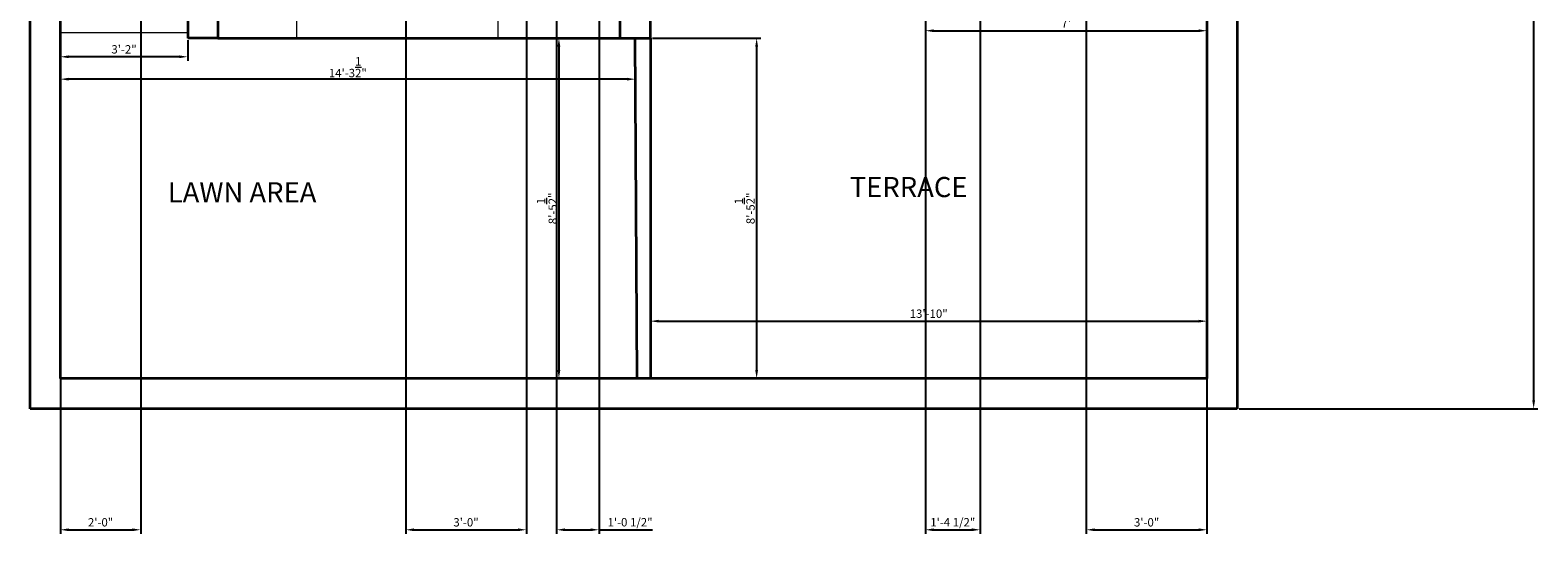
# Model space of a CAD drawing. Units: inches. Extents: x 2178 to 2667, y 1439 to 2239.
# Tile 1 of 5: x 2218 to 2667, y 1439 to 1590. Entities that reach past the tile are written whole.
import ezdxf

# ---------------------------------------------------------------- set-up
doc = ezdxf.new("R2010")
doc.units = ezdxf.units.IN
for name, color, linetype, lineweight in [('A-ANNO-DIMS', 2, 'Continuous', 18), ('A-AREA-IDEN', 7, 'Continuous', 18), ('A-FLOR-PATT', 252, 'Continuous', 13), ('A-GLAZ', 4, 'Continuous', 18), ('A-WALL', 7, 'Continuous', 35)]:
    doc.layers.add(name, color=color, linetype=linetype, lineweight=lineweight)
doc.styles.get("Standard").update_dxf_attribs({"font": 'arial.ttf'})
doc.dimstyles.new('Copy of ISO-25', dxfattribs={"dimtxt": 2.5, "dimasz": 2.5, "dimexe": 1.25, "dimexo": 0.625, "dimtad": 1, "dimdec": 1, "dimlunit": 4, "dimtxsty": 'Standard', "dimcen": 2.5, "dimadec": 0, "dimazin": 0, "dimtfac": 1, "dimtdec": 1, "dimtmove": 0, "dimatfit": 3, "dimfxl": 1, "dimarcsym": 0})

# ---------------------------------------------------------------- blocks, each defined once
blk = doc.blocks.new('*D25')
at = {"layer": 'A-ANNO-DIMS', "color": 0, "lineweight": -2, "transparency": 16777216}
for p, q in [((2226.53, 1586.91), (2226.53, 1574.05)), ((2398.03, 1586.91), (2398.03, 1574.05)), ((2395.53, 1575.3), (2229.03, 1575.3))]:
    blk.add_line(p, q, dxfattribs=at)
at = {"layer": 'A-ANNO-DIMS', "color": 0, "transparency": 16777216}
for points in [[(2229.03, 1575.72), (2229.03, 1574.89), (2226.53, 1575.3)], [(2395.53, 1575.72), (2395.53, 1574.89), (2398.03, 1575.3)]]:
    blk.add_solid(points, dxfattribs=at)
at = {"layer": 'Defpoints', "color": 0, "transparency": 16777216}
for p in [(2226.53, 1587.53), (2398.03, 1587.53), (2226.53, 1575.3)]:
    blk.add_point(p, dxfattribs=at)
at = {"layer": 'A-ANNO-DIMS', "color": 0, "transparency": 16777216, "insert": (2312.28, 1578.88), "char_height": 2.5, "attachment_point": 5}
blk.add_mtext('14\'-3{\\H1x;\\S1/2;}"', dxfattribs=at)
blk = doc.blocks.new('*D26')
at = {"layer": 'A-ANNO-DIMS', "color": 0, "lineweight": -2, "transparency": 16777216}
for p, q in [((2397.4, 1587.53), (2373.98, 1587.53)), ((2375.23, 1585.03), (2375.23, 1488.53)), ((2397.9, 1486.03), (2373.98, 1486.03))]:
    blk.add_line(p, q, dxfattribs=at)
at = {"layer": 'A-ANNO-DIMS', "color": 0, "transparency": 16777216}
for points in [[(2374.82, 1585.03), (2375.65, 1585.03), (2375.23, 1587.53)], [(2374.82, 1488.53), (2375.65, 1488.53), (2375.23, 1486.03)]]:
    blk.add_solid(points, dxfattribs=at)
at = {"layer": 'Defpoints', "color": 0, "transparency": 16777216}
for p in [(2398.03, 1587.53), (2375.23, 1486.03), (2398.53, 1486.03)]:
    blk.add_point(p, dxfattribs=at)
at = {"layer": 'A-ANNO-DIMS', "color": 0, "transparency": 16777216, "insert": (2371.66, 1536.78), "char_height": 2.5, "attachment_point": 5, "rotation": 90}
blk.add_mtext('8\'-5{\\H1x;\\S1/2;}"', dxfattribs=at)
blk = doc.blocks.new('*D27')
at = {"layer": 'A-ANNO-DIMS', "color": 0, "lineweight": -2, "transparency": 16777216}
for p, q in [((2402.53, 1486.66), (2402.53, 1504.39)), ((2405.03, 1503.14), (2566.03, 1503.14)), ((2568.53, 1486.66), (2568.53, 1504.39))]:
    blk.add_line(p, q, dxfattribs=at)
at = {"layer": 'A-ANNO-DIMS', "color": 0, "transparency": 16777216}
for points in [[(2405.03, 1503.56), (2405.03, 1502.73), (2402.53, 1503.14)], [(2566.03, 1503.56), (2566.03, 1502.73), (2568.53, 1503.14)]]:
    blk.add_solid(points, dxfattribs=at)
at = {"layer": 'Defpoints', "color": 0, "transparency": 16777216}
for p in [(2568.53, 1503.14), (2402.53, 1486.03), (2568.53, 1486.03)]:
    blk.add_point(p, dxfattribs=at)
at = {"layer": 'A-ANNO-DIMS', "color": 0, "transparency": 16777216, "insert": (2485.53, 1505.05), "char_height": 2.5, "attachment_point": 5}
blk.add_mtext('13\'-10"', dxfattribs=at)
blk = doc.blocks.new('*D28')
at = {"layer": 'A-ANNO-DIMS', "color": 0, "lineweight": -2, "transparency": 16777216}
for p, q in [((2403.15, 1587.53), (2435.47, 1587.53)), ((2434.22, 1585.03), (2434.22, 1488.53)), ((2403.15, 1486.03), (2435.47, 1486.03))]:
    blk.add_line(p, q, dxfattribs=at)
at = {"layer": 'A-ANNO-DIMS', "color": 0, "transparency": 16777216}
for points in [[(2433.8, 1585.03), (2434.63, 1585.03), (2434.22, 1587.53)], [(2433.8, 1488.53), (2434.63, 1488.53), (2434.22, 1486.03)]]:
    blk.add_solid(points, dxfattribs=at)
at = {"layer": 'Defpoints', "color": 0, "transparency": 16777216}
for p in [(2402.53, 1587.53), (2402.53, 1486.03), (2434.22, 1486.03)]:
    blk.add_point(p, dxfattribs=at)
at = {"layer": 'A-ANNO-DIMS', "color": 0, "transparency": 16777216, "insert": (2430.64, 1536.78), "char_height": 2.5, "attachment_point": 5, "rotation": 90}
blk.add_mtext('8\'-5{\\H1x;\\S1/2;}"', dxfattribs=at)
blk = doc.blocks.new('*D31')
at = {"layer": 'A-ANNO-DIMS', "color": 0, "lineweight": -2, "transparency": 16777216}
for p, q in [((2484.53, 1600.12), (2484.53, 1588.5)), ((2568.53, 1600.12), (2568.53, 1588.5)), ((2487.03, 1589.75), (2566.03, 1589.75))]:
    blk.add_line(p, q, dxfattribs=at)
at = {"layer": 'A-ANNO-DIMS', "color": 0, "transparency": 16777216}
for points in [[(2487.03, 1590.17), (2487.03, 1589.33), (2484.53, 1589.75)], [(2566.03, 1590.17), (2566.03, 1589.33), (2568.53, 1589.75)]]:
    blk.add_solid(points, dxfattribs=at)
at = {"layer": 'Defpoints', "color": 0, "transparency": 16777216}
for p in [(2484.53, 1600.74), (2568.53, 1600.74), (2568.53, 1589.75)]:
    blk.add_point(p, dxfattribs=at)
at = {"layer": 'A-ANNO-DIMS', "color": 0, "transparency": 16777216, "insert": (2526.53, 1591.63), "char_height": 2.5, "attachment_point": 5}
blk.add_mtext("7'", dxfattribs=at)
blk = doc.blocks.new('*D40')
at = {"layer": 'A-ANNO-DIMS', "color": 0, "lineweight": -2, "transparency": 16777216}
for p, q in [((2226.53, 1586.91), (2226.53, 1580.73)), ((2264.53, 1586.91), (2264.53, 1580.73)), ((2262.03, 1581.98), (2229.03, 1581.98))]:
    blk.add_line(p, q, dxfattribs=at)
at = {"layer": 'A-ANNO-DIMS', "color": 0, "transparency": 16777216}
for points in [[(2229.03, 1582.4), (2229.03, 1581.57), (2226.53, 1581.98)], [(2262.03, 1582.4), (2262.03, 1581.57), (2264.53, 1581.98)]]:
    blk.add_solid(points, dxfattribs=at)
at = {"layer": 'Defpoints', "color": 0, "transparency": 16777216}
for p in [(2226.53, 1587.53), (2264.53, 1587.53), (2226.53, 1581.98)]:
    blk.add_point(p, dxfattribs=at)
at = {"layer": 'A-ANNO-DIMS', "color": 0, "transparency": 16777216, "insert": (2245.53, 1583.88), "char_height": 2.5, "attachment_point": 5}
blk.add_mtext('3\'-2"', dxfattribs=at)
blk = doc.blocks.new('*D41')
at = {"layer": 'A-ANNO-DIMS', "color": 0, "lineweight": -2, "transparency": 16777216}
for p, q in [((2578.15, 2197.03), (2667.22, 2197.03)), ((2665.97, 2194.53), (2665.97, 1479.53)), ((2578.15, 1477.03), (2667.22, 1477.03))]:
    blk.add_line(p, q, dxfattribs=at)
at = {"layer": 'A-ANNO-DIMS', "color": 0, "transparency": 16777216}
for points in [[(2665.56, 2194.53), (2666.39, 2194.53), (2665.97, 2197.03)], [(2665.56, 1479.53), (2666.39, 1479.53), (2665.97, 1477.03)]]:
    blk.add_solid(points, dxfattribs=at)
at = {"layer": 'Defpoints', "color": 0, "transparency": 16777216}
for p in [(2577.53, 2197.03), (2577.53, 1477.03), (2665.97, 1477.03)]:
    blk.add_point(p, dxfattribs=at)
at = {"layer": 'A-ANNO-DIMS', "color": 0, "transparency": 16777216, "insert": (2664.07, 1837.03), "char_height": 2.5, "attachment_point": 5, "rotation": 90}
blk.add_mtext("60'", dxfattribs=at)
blk = doc.blocks.new('*D57')
at = {"layer": 'A-ANNO-DIMS', "color": 0, "lineweight": -2, "transparency": 16777216}
for p, q in [((2374.53, 2119.41), (2374.53, 1439.68)), ((2387.22, 2119.41), (2387.22, 1439.68)), ((2377.03, 1440.93), (2384.72, 1440.93)), ((2387.22, 1440.93), (2403.2, 1440.93))]:
    blk.add_line(p, q, dxfattribs=at)
at = {"layer": 'A-ANNO-DIMS', "color": 0, "transparency": 16777216}
for points in [[(2377.03, 1441.35), (2377.03, 1440.52), (2374.53, 1440.93)], [(2384.72, 1441.35), (2384.72, 1440.52), (2387.22, 1440.93)]]:
    blk.add_solid(points, dxfattribs=at)
at = {"layer": 'Defpoints', "color": 0, "transparency": 16777216}
for p in [(2374.53, 2120.03), (2387.22, 2120.03), (2387.22, 1440.93)]:
    blk.add_point(p, dxfattribs=at)
at = {"layer": 'A-ANNO-DIMS', "color": 0, "transparency": 16777216, "insert": (2396.46, 1442.85), "char_height": 2.5, "attachment_point": 5}
blk.add_mtext('1\'-0 1/2"', dxfattribs=at)
blk = doc.blocks.new('*D58')
at = {"layer": 'A-ANNO-DIMS', "color": 0, "lineweight": -2, "transparency": 16777216}
for p, q in [((2484.53, 1740.12), (2484.53, 1439.68)), ((2500.89, 1740.12), (2500.89, 1439.68)), ((2487.03, 1440.93), (2498.39, 1440.93))]:
    blk.add_line(p, q, dxfattribs=at)
at = {"layer": 'A-ANNO-DIMS', "color": 0, "transparency": 16777216}
for points in [[(2487.03, 1441.35), (2487.03, 1440.52), (2484.53, 1440.93)], [(2498.39, 1441.35), (2498.39, 1440.52), (2500.89, 1440.93)]]:
    blk.add_solid(points, dxfattribs=at)
at = {"layer": 'Defpoints', "color": 0, "transparency": 16777216}
for p in [(2484.53, 1740.74), (2500.89, 1740.74), (2500.89, 1440.93)]:
    blk.add_point(p, dxfattribs=at)
at = {"layer": 'A-ANNO-DIMS', "color": 0, "transparency": 16777216, "insert": (2492.71, 1442.85), "char_height": 2.5, "attachment_point": 5}
blk.add_mtext('1\'-4 1/2"', dxfattribs=at)
blk = doc.blocks.new('*D67')
at = {"layer": 'A-ANNO-DIMS', "color": 0, "lineweight": -2, "transparency": 16777216}
for p, q in [((2226.53, 2022.41), (2226.53, 1439.68)), ((2250.53, 2022.41), (2250.53, 1439.68)), ((2229.03, 1440.93), (2248.03, 1440.93))]:
    blk.add_line(p, q, dxfattribs=at)
at = {"layer": 'A-ANNO-DIMS', "color": 0, "transparency": 16777216}
for points in [[(2229.03, 1441.35), (2229.03, 1440.52), (2226.53, 1440.93)], [(2248.03, 1441.35), (2248.03, 1440.52), (2250.53, 1440.93)]]:
    blk.add_solid(points, dxfattribs=at)
at = {"layer": 'Defpoints', "color": 0, "transparency": 16777216}
for p in [(2226.53, 2023.03), (2250.53, 2023.03), (2250.53, 1440.93)]:
    blk.add_point(p, dxfattribs=at)
at = {"layer": 'A-ANNO-DIMS', "color": 0, "transparency": 16777216, "insert": (2238.53, 1442.84), "char_height": 2.5, "attachment_point": 5}
blk.add_mtext('2\'-0"', dxfattribs=at)
blk = doc.blocks.new('*D69')
at = {"layer": 'A-ANNO-DIMS', "color": 0, "lineweight": -2, "transparency": 16777216}
for p, q in [((2329.53, 2022.41), (2329.53, 1439.68)), ((2365.53, 2001.3), (2365.53, 1439.68)), ((2332.03, 1440.93), (2363.03, 1440.93))]:
    blk.add_line(p, q, dxfattribs=at)
at = {"layer": 'A-ANNO-DIMS', "color": 0, "transparency": 16777216}
for points in [[(2332.03, 1441.35), (2332.03, 1440.52), (2329.53, 1440.93)], [(2363.03, 1441.35), (2363.03, 1440.52), (2365.53, 1440.93)]]:
    blk.add_solid(points, dxfattribs=at)
at = {"layer": 'Defpoints', "color": 0, "transparency": 16777216}
for p in [(2329.53, 2023.03), (2365.53, 2001.92), (2365.53, 1440.93)]:
    blk.add_point(p, dxfattribs=at)
at = {"layer": 'A-ANNO-DIMS', "color": 0, "transparency": 16777216, "insert": (2347.53, 1442.84), "char_height": 2.5, "attachment_point": 5}
blk.add_mtext('3\'-0"', dxfattribs=at)
blk = doc.blocks.new('*D73')
at = {"layer": 'A-ANNO-DIMS', "color": 0, "lineweight": -2, "transparency": 16777216}
for p, q in [((2568.53, 2187.41), (2568.53, 1439.68)), ((2532.53, 2128.41), (2532.53, 1439.68)), ((2535.03, 1440.93), (2566.03, 1440.93))]:
    blk.add_line(p, q, dxfattribs=at)
at = {"layer": 'A-ANNO-DIMS', "color": 0, "transparency": 16777216}
for points in [[(2535.03, 1441.35), (2535.03, 1440.52), (2532.53, 1440.93)], [(2566.03, 1441.35), (2566.03, 1440.52), (2568.53, 1440.93)]]:
    blk.add_solid(points, dxfattribs=at)
at = {"layer": 'Defpoints', "color": 0, "transparency": 16777216}
for p in [(2568.53, 2188.03), (2532.53, 2129.03), (2568.53, 1440.93)]:
    blk.add_point(p, dxfattribs=at)
at = {"layer": 'A-ANNO-DIMS', "color": 0, "transparency": 16777216, "insert": (2550.53, 1442.84), "char_height": 2.5, "attachment_point": 5}
blk.add_mtext('3\'-0"', dxfattribs=at)

msp = doc.modelspace()

# ---------------------------------------------------------------- linework, layer by layer
at = {"layer": 'A-FLOR-PATT'}
msp.add_lwpolyline([(2226.53, 1728.32), (2264.53, 1728.32), (2264.53, 1589.16), (2226.53, 1589.16)], close=True, dxfattribs=at)
at = {"layer": 'A-GLAZ'}
for p, q in [((2297.04, 1587.53), (2297.04, 1596.53)), ((2357.04, 1596.53), (2357.04, 1587.53))]:
    msp.add_line(p, q, dxfattribs=at)
at = {"layer": 'A-WALL'}
for p, q in [((2217.53, 1477.03), (2217.53, 2197.03)), ((2577.53, 2197.03), (2577.53, 1477.03)), ((2226.53, 1486.03), (2226.53, 1796.03)), ((2568.53, 1740.74), (2568.53, 1486.03)), ((2264.53, 1683.53), (2264.53, 1587.53)), ((2273.53, 1683.53), (2273.53, 1587.53)), ((2393.53, 1587.53), (2393.53, 1683.53)), ((2402.53, 1587.53), (2402.53, 1683.53)), ((2273.53, 1596.53), (2273.53, 1587.53)), ((2393.53, 1587.53), (2393.53, 1596.53)), ((2273.53, 1587.53), (2264.53, 1587.53)), ((2273.53, 1587.53), (2393.53, 1587.53)), ((2273.53, 1587.53), (2297.04, 1587.53)), ((2393.53, 1587.53), (2402.53, 1587.53)), ((2398.53, 1486.03), (2398.03, 1587.53)), ((2402.53, 1587.53), (2402.53, 1486.03)), ((2568.53, 1486.03), (2226.53, 1486.03)), ((2402.53, 1486.03), (2398.53, 1486.03)), ((2402.53, 1486.03), (2398.53, 1486.03)), ((2577.53, 1477.03), (2217.53, 1477.03))]:
    msp.add_line(p, q, dxfattribs=at)

# ---------------------------------------------------------------- texts
at = {"layer": 'A-AREA-IDEN'}
for s, p in [('LAWN AREA', (2258.57, 1538.57)), ('TERRACE', (2461.98, 1540.14))]:
    msp.add_text(s, height=6, dxfattribs=at).set_placement(p)

# ---------------------------------------------------------------- dimensions: what is measured, and where the dimension line sits
at = {"layer": 'A-ANNO-DIMS'}
for base, p1, p2, picture, middle in [((2665.97, 1477.03), (2577.53, 2197.03), (2577.53, 1477.03), '*D41', (2664.07, 1837.03)), ((2375.23, 1486.03), (2398.03, 1587.53), (2398.53, 1486.03), '*D26', (2371.66, 1536.78)), ((2434.22, 1486.03), (2402.53, 1587.53), (2402.53, 1486.03), '*D28', (2430.64, 1536.78))]:
    dim = msp.add_linear_dim(base=base, p1=p1, p2=p2, angle=90, dimstyle='Copy of ISO-25', override={"dimclrd": 0, "dimclre": 0, "dimclrt": 0}, dxfattribs=at)
    dim.commit()
    dim.dimension.update_dxf_attribs({"geometry": picture, "text_midpoint": middle})
for base, p1, p2, override, picture, middle in [((2568.53, 1440.93), (2532.53, 2129.03), (2568.53, 2188.03), {"dimdec": 1, "dimlfac": 1, "dimrnd": 0, "dimzin": 1, "dimdsep": 46, "dimlunit": 4, "dimfrac": 2}, '*D73', (2550.53, 1442.84)), ((2387.22, 1440.93), (2374.53, 2120.03), (2387.22, 2120.03), {"dimdec": 1, "dimlfac": 1, "dimrnd": 0, "dimzin": 1, "dimdsep": 46, "dimlunit": 4, "dimfrac": 2}, '*D57', (2396.46, 1442.85)), ((2250.53, 1440.93), (2226.53, 2023.03), (2250.53, 2023.03), {"dimdec": 1, "dimlfac": 1, "dimrnd": 0, "dimzin": 1, "dimdsep": 46, "dimlunit": 4, "dimfrac": 2}, '*D67', (2238.53, 1442.84)), ((2365.53, 1440.93), (2329.53, 2023.03), (2365.53, 2001.92), {"dimdec": 1, "dimlfac": 1, "dimrnd": 0, "dimzin": 1, "dimdsep": 46, "dimlunit": 4, "dimfrac": 2}, '*D69', (2347.53, 1442.84)), ((2500.89, 1440.93), (2484.53, 1740.74), (2500.89, 1740.74), {"dimdec": 1, "dimlfac": 1, "dimrnd": 0, "dimzin": 1, "dimdsep": 46, "dimlunit": 4, "dimfrac": 2}, '*D58', (2492.71, 1442.85)), ((2568.53, 1589.75), (2484.53, 1600.74), (2568.53, 1600.74), {"dimclrd": 0, "dimclre": 0, "dimclrt": 0}, '*D31', (2526.53, 1591.63)), ((2226.53, 1575.3), (2398.03, 1587.53), (2226.53, 1587.53), {"dimclrd": 0, "dimclre": 0, "dimclrt": 0}, '*D25', (2312.28, 1578.88)), ((2226.53, 1581.98), (2264.53, 1587.53), (2226.53, 1587.53), {"dimclrd": 0, "dimclre": 0, "dimclrt": 0}, '*D40', (2245.53, 1583.88)), ((2568.53, 1503.14), (2402.53, 1486.03), (2568.53, 1486.03), {"dimclrd": 0, "dimclre": 0, "dimclrt": 0}, '*D27', (2485.53, 1505.05))]:
    dim = msp.add_linear_dim(base=base, p1=p1, p2=p2, dimstyle='Copy of ISO-25', override=override, dxfattribs=at)
    dim.commit()
    dim.dimension.update_dxf_attribs({"geometry": picture, "text_midpoint": middle})

doc.saveas('drawing.dxf')
